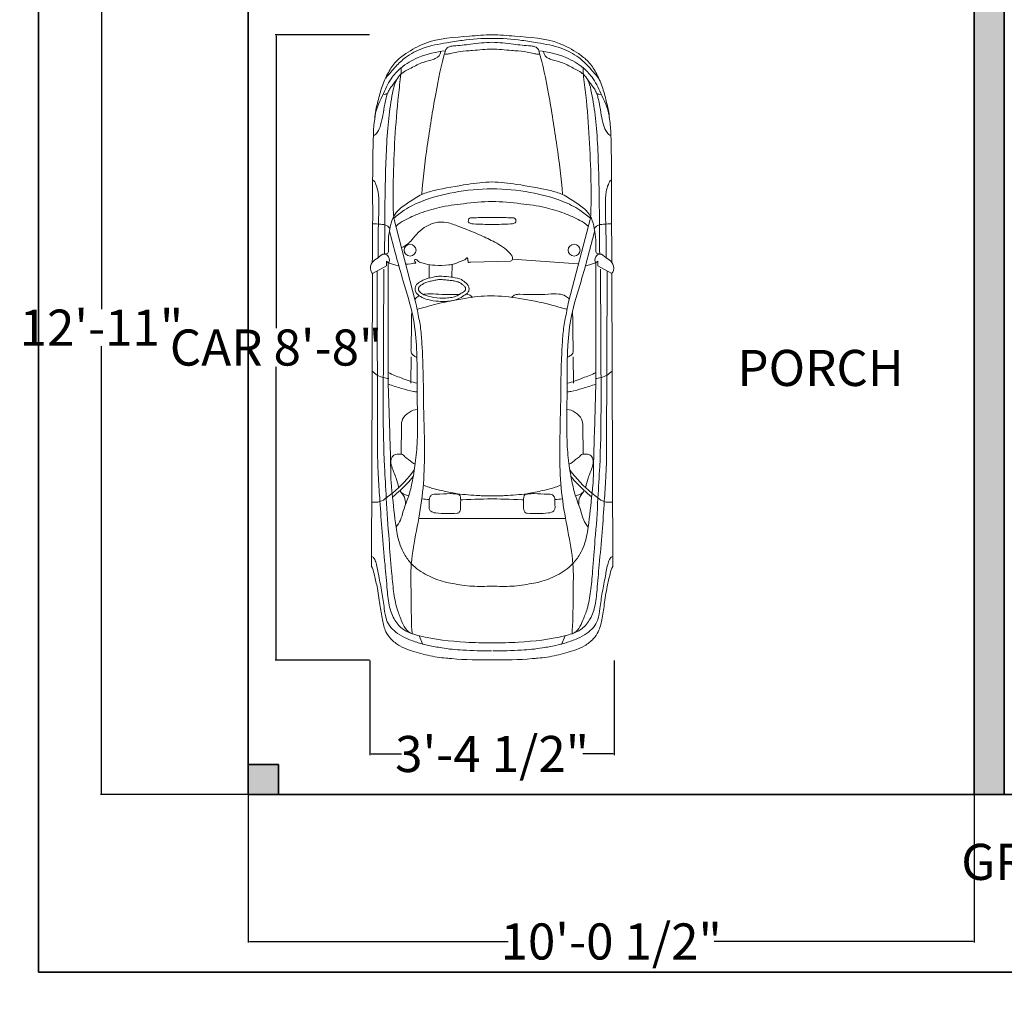
# Model space of a CAD drawing. Units: inches. Extents: x 717 to 1167, y 2046 to 2594.
# Tile 1 of 6: x 717 to 880, y 2046 to 2208. Entities that reach past the tile are written whole.
import ezdxf

# ---------------------------------------------------------------- set-up
doc = ezdxf.new("R2010")
doc.units = ezdxf.units.IN
doc.header["$MEASUREMENT"] = 0
for name, color, linetype, lineweight in [('A-ANNO-DIMS', 2, 'Continuous', 18), ('A-ANNO-TEXT', 7, 'Continuous', 25), ('A-ANNO-TTLB', 7, 'Continuous', 35), ('A-AREA-IDEN', 7, 'Continuous', 18), ('A-COLS', 7, 'Continuous', 35), ('A-COLS-PATT', 140, 'Continuous', 13), ('A-EQPM-VEHI', 8, 'Continuous', 18), ('A-WALL', 7, 'Continuous', 35), ('A-WALL-PATT', 140, 'Continuous', 13)]:
    doc.layers.add(name, color=color, linetype=linetype, lineweight=lineweight)
doc.styles.get("Standard").update_dxf_attribs({"font": 'arial.ttf'})
doc.dimstyles.get("Standard").update_dxf_attribs({"dimtxt": 6, "dimasz": 0.18, "dimexe": 0.18, "dimexo": 0.0625, "dimgap": 0.09, "dimtad": 0, "dimtih": 1, "dimtoh": 1, "dimdec": 1, "dimzin": 0, "dimdsep": 46, "dimlunit": 3, "dimtxsty": 'Standard', "dimcen": 0.09, "dimadec": 0, "dimazin": 0, "dimtfac": 1, "dimtdec": 1, "dimtofl": 0, "dimtmove": 0, "dimatfit": 3, "dimfxl": 1, "dimtolj": 1, "dimtzin": 0, "dimarcsym": 0})

# ---------------------------------------------------------------- blocks, each defined once
blk = doc.blocks.new('A$C242571DA')
for p, q in [((1659.9, 1632), (1714.3, 1732.5)), ((1699.9, 1699.4), (2984.7, 1695.8)), ((1714.3, 1732.5), (3817.1, 1739.9)), ((1638.3, 1618.5), (1625.1, 1632)), ((1625.1, 1632), (1659.9, 1632)), ((1681.8, 1651.6), (2695.2, 1655.3)), ((1317.4, 1579.7), (1909.8, 1424.9)), ((1638.3, 1618.5), (2503.3, 1618.5)), ((1659.9, 1548.1), (1638.3, 1618.5)), ((2503.3, 1618.5), (2861.6, 1607.5)), ((1644, 1489.1), (1610.4, 1020.2)), ((3007.2, 1526.5), (2808.1, 1525.2)), ((2311.9, 1454.3), (2500.6, 1456.9)), ((3474.6, 1401.1), (3474.6, 843)), ((4315.2, 1398), (4377.3, 1370.5)), ((1626.1, 1006.5), (1632.8, 719.7)), ((3474.6, 345.6), (3474.6, 903.8)), ((1740.2, 584.9), (1649.3, 586.9)), ((1746.1, 420.6), (1649.3, 420.6)), ((4315.2, 348.7), (4377.3, 376.3)), ((1317.4, 167), (1909.8, 321.9)), ((2311.9, 292.5), (2500.6, 289.8)), ((3007.2, 220.3), (2808.1, 221.6)), ((1659.9, 198.7), (1638.3, 128.2)), ((1638.3, 128.2), (1625.1, 114.7)), ((1625.1, 114.7), (1659.9, 114.7)), ((1638.3, 128.2), (2503.3, 128.2)), ((1659.9, 114.7), (1714.3, 14.2)), ((1681.8, 95.1), (2695.2, 91.4)), ((2503.3, 128.2), (2861.6, 139.2)), ((1699.9, 47.3), (2984.7, 51)), ((1714.3, 14.2), (3817.1, 6.9))]:
    blk.add_line(p, q)
for centre in [(1546.4, 1462.5), (1546.4, 284.2)]:
    blk.add_ellipse(centre, major_axis=(0, 42.9), ratio=0.983266, start_param=4.712389, end_param=10.995574)
for points, knots in [([(0, 873.4), (0, 927.8), (15.6, 1088.6), (25.5, 1309.8), (120.7, 1476.4), (189.2, 1569), (273.5, 1623.1), (369.9, 1666.3), (483, 1694.7), (561.3, 1714.9), (604.6, 1715.7)], [0, 0, 0, 0, 0.16039, 0.479033, 0.632967, 0.722015, 0.817474, 0.927562, 1.03733, 1.167094, 1.167094, 1.167094, 1.167094]), ([(604.6, 1715.7), (545.5, 1714.5), (448.5, 1664.6), (320.8, 1610.6), (225.4, 1521.2), (147.3, 1390.5), (121.7, 1275.2), (113.6, 1208.7)], [0, 0, 0, 0, 0.1772572, 0.3124951, 0.4151678, 0.5597243, 0.7575412, 0.7575412, 0.7575412, 0.7575412]), ([(722.7, 1726.6), (720.8, 1714.9), (694.5, 1689.9), (643, 1671.8), (573.6, 1655.4), (508.5, 1647), (455.2, 1634.7), (428.7, 1627.3), (416.9, 1624.1)], [0, 0, 0, 0, 0.034703, 0.0959761, 0.1659336, 0.2471559, 0.2929944, 0.3295918, 0.3295918, 0.3295918, 0.3295918]), ([(604.6, 1715.7), (642.1, 1723.4), (788.5, 1729.2), (1039.3, 1732.2), (1344.5, 1729.9), (1542, 1733.1), (1633.8, 1733.7)], [0, 0, 0, 0, 0.114897, 0.437061, 0.754269, 1.029686, 1.029686, 1.029686, 1.029686]), ([(1043.6, 1729.2), (1048.6, 1717.9), (1080.9, 1704.2), (1138.6, 1687.6), (1237.7, 1685.6), (1394.7, 1691.3), (1521.7, 1692.4), (1601.5, 1692.7)], [0, 0, 0, 0, 0.0364992, 0.0923739, 0.1867837, 0.3273982, 0.5667068, 0.5667068, 0.5667068, 0.5667068]), ([(1356.8, 1732.2), (1357.1, 1712.8), (1360, 1678.8), (1363.9, 1630.5), (1383.3, 1613.5), (1391, 1607.2)], [0, 0, 0, 0, 1.462159, 2.651105, 3.386321, 3.386321, 3.386321, 3.386321]), ([(1714.3, 1732.5), (1707.7, 1737.6), (1683.3, 1753), (1628.7, 1741.2), (1605.6, 1691.5), (1561.7, 1652.4), (1594.1, 1610.3), (1627.9, 1608.3), (1638.3, 1618.5)], [0, 0, 0, 0, 0.024864, 0.0846267, 0.1362471, 0.1900683, 0.2245199, 0.2681841, 0.2681841, 0.2681841, 0.2681841]), ([(2414.7, 1735), (2424.9, 1723.3), (2447.2, 1698.8), (2461.2, 1657.6), (2468.1, 1629), (2468, 1616.1)], [1.808086, 1.808086, 1.808086, 1.808086, 2.918874, 4.131288, 5.10151, 5.10151, 5.10151, 5.10151]), ([(3356.5, 1739.4), (3354.9, 1719.2), (3360.8, 1678.2), (3324, 1631.5), (3255.4, 1544.3), (3187.1, 1476.2), (3125.2, 1432.2)], [0, 0, 0, 0, 0.0597371, 0.1139981, 0.1672498, 0.3938869, 0.3938869, 0.3938869, 0.3938869]), ([(3745.3, 1736.8), (3748.5, 1730.1), (3764.2, 1717.1), (3811.5, 1698.6), (3894.7, 1686.7), (4002.9, 1663.2), (4107.9, 1648.7), (4195.8, 1638.3), (4258.6, 1603.2), (4302.1, 1549.7), (4339.9, 1483.8), (4365.2, 1407.6), (4389.6, 1324.4), (4397.9, 1266.9), (4401.8, 1235.2)], [0, 0, 0, 0, 0.0219205, 0.0572122, 0.1522539, 0.2718866, 0.3894011, 0.4710097, 0.5346344, 0.5986698, 0.6733118, 0.758696, 0.8351341, 0.9293726, 0.9293726, 0.9293726, 0.9293726]), ([(3817.1, 1739.9), (3833.2, 1729.7), (3882.9, 1718.2), (3973.3, 1695.2), (4085.1, 1680.5), (4193.8, 1662.8), (4280.6, 1644.3), (4343.9, 1598.1), (4390, 1540.3), (4427.4, 1448.7), (4457.8, 1336.6), (4475.7, 1233.4), (4478.4, 1175.1), (4479.3, 1161.6)], [0, 0, 0, 0, 0.056668, 0.14946, 0.28161, 0.392935, 0.481686, 0.542967, 0.622845, 0.69797, 0.833643, 0.965665, 1.00577, 1.00577, 1.00577, 1.00577]), ([(310.7, 1637.3), (282.5, 1613.7), (230.1, 1569.9), (148.7, 1486.2), (84.8, 1361.3), (60, 1219), (32.6, 1054.3), (25.1, 944.9), (25.1, 873.4)], [0, 0, 0, 0, 0.1095129, 0.2035347, 0.3452507, 0.5161382, 0.6275464, 0.8383798, 0.8383798, 0.8383798, 0.8383798]), ([(426.8, 1656.7), (428.5, 1646.6), (426.9, 1625), (399.8, 1616.6), (368.1, 1593.9), (328, 1564.6), (271.6, 1523.9), (237, 1451.9), (196.2, 1376.7), (183.8, 1314.9), (170, 1279.6), (157.2, 1254.2), (133.3, 1244.4), (118.6, 1242.9)], [0, 0, 0, 0, 0.0304541, 0.0502818, 0.0786089, 0.1479133, 0.1986294, 0.2831705, 0.3780326, 0.4523267, 0.4667809, 0.4902599, 0.5347198, 0.5347198, 0.5347198, 0.5347198]), ([(323.7, 1557.5), (344.8, 1571.9), (400.4, 1585.1), (516, 1606.8), (680.3, 1625.8), (885.4, 1635.7), (1116.8, 1642.2), (1346.1, 1644.2), (1504.7, 1644.7), (1574, 1645.7)], [0, 0, 0, 0, 0.076148, 0.165903, 0.355672, 0.569871, 0.782325, 1.050047, 1.257936, 1.257936, 1.257936, 1.257936]), ([(1574, 1645.7), (1572.9, 1638), (1574.1, 1622), (1559.9, 1618.7), (1555.2, 1617.8)], [0, 0, 0, 0, 0.02274132, 0.03717479, 0.03717479, 0.03717479, 0.03717479]), ([(2695.2, 1655.3), (2829.9, 1655.3), (3041.2, 1651.4), (3351.3, 1630.7), (3527.5, 1623.2), (3626.6, 1612)], [0, 0, 0, 0, 0.4042759, 0.6333827, 0.9326252, 0.9326252, 0.9326252, 0.9326252]), ([(2984.7, 1695.8), (3051, 1695.6), (3172.1, 1691.3), (3367.4, 1677.6), (3575.2, 1664.3), (3788.2, 1643.6), (3968, 1628.1), (4103.8, 1616.8), (4203.6, 1578.1), (4271.8, 1519.5), (4300.6, 1452.1), (4341.7, 1305.3), (4361.8, 1111.2), (4367.5, 936.8), (4367.5, 873.4)], [0, 0, 0, 0, 0.198873, 0.363323, 0.587433, 0.823543, 1.004622, 1.129816, 1.230113, 1.320655, 1.388577, 1.443334, 1.771447, 1.958652, 1.958652, 1.958652, 1.958652]), ([(1317.4, 1579.7), (1227.8, 1586.1), (1036, 1584.8), (741.2, 1572.5), (486.1, 1553.3), (333.3, 1534.3), (283.3, 1528.5)], [0, 0, 0, 0, 0.269375, 0.574535, 0.885339, 1.036319, 1.036319, 1.036319, 1.036319]), ([(1555.2, 1617.8), (1527.7, 1617.8), (1472.5, 1620.4), (1392.7, 1608.8), (1318.5, 1591), (1249.4, 1545.5), (1201.4, 1466.7), (1142.8, 1385.7), (1104.8, 1240.4), (1076, 1072.3), (1056.4, 932.4), (1056.4, 873.4)], [0, 0, 0, 0, 0.082256, 0.165174, 0.241383, 0.30939, 0.405348, 0.511507, 0.603349, 0.843635, 1.017671, 1.017671, 1.017671, 1.017671]), ([(1317.4, 1579.7), (1296.6, 1555.5), (1247.9, 1494.4), (1177.6, 1350.5), (1124.2, 1137.4), (1105.5, 964.9), (1105.5, 873.4)], [0, 0, 0, 0, 0.0947759, 0.2311242, 0.4700259, 0.7400315, 0.7400315, 0.7400315, 0.7400315]), ([(1372.8, 1563.1), (1357.2, 1545), (1321.6, 1490.1), (1277, 1385.7), (1232.8, 1244.2), (1211.1, 1069.4), (1196.8, 942.4), (1196.8, 873.4)], [0, 0, 0, 0, 0.0708922, 0.1925846, 0.3348457, 0.5072814, 0.7109928, 0.7109928, 0.7109928, 0.7109928]), ([(3535.9, 1563.1), (3520.1, 1550.9), (3484.4, 1526.1), (3408.2, 1510.9), (3323.4, 1473.1), (3207.9, 1445), (3072.6, 1422.2), (2866.9, 1404.6), (2626.4, 1412.9), (2396.7, 1410.8), (2200.9, 1416.9), (2001.3, 1438.2), (1732.1, 1525.9), (1527.9, 1578.9), (1407.5, 1610.7)], [0, 0, 0, 0, 0.05975, 0.126928, 0.230034, 0.336675, 0.482225, 0.641324, 0.954906, 1.203173, 1.330375, 1.542773, 1.802261, 2.175545, 2.175545, 2.175545, 2.175545]), ([(2424, 1618.7), (2441.5, 1589.9), (2464.2, 1518.9), (2495.4, 1450.9), (2501.6, 1411.3)], [0, 0, 0, 0, 0.1000351, 0.2184418, 0.2184418, 0.2184418, 0.2184418]), ([(2507.7, 1618.4), (2521, 1587.7), (2536.6, 1527.1), (2559.6, 1458.5), (2563.3, 1420.6), (2563.8, 1411.4)], [0, 0, 0, 0, 2.528586, 4.711885, 5.408215, 5.408215, 5.408215, 5.408215]), ([(2861.6, 1607.5), (2921.1, 1607.3), (3047.2, 1600.8), (3191.4, 1602), (3356.6, 1584.1), (3498.3, 1570.6), (3623.2, 1549.4), (3664.1, 1533.3)], [0, 0, 0, 0, 0.1783018, 0.3787173, 0.431954, 0.6762374, 0.8077184, 0.8077184, 0.8077184, 0.8077184]), ([(3248.1, 1545.2), (3226.9, 1550.4), (3176.1, 1562.1), (3113.7, 1592.9), (3052.6, 1605.3), (3010.4, 1578.8), (3010.3, 1545.3), (3010.3, 1515.9), (3033.7, 1500.1), (3052.6, 1465.2), (3078.9, 1443.5), (3084, 1424.4)], [0, 0, 0, 0, 0.0655106, 0.1550445, 0.2094604, 0.2438604, 0.287164, 0.3001388, 0.3275984, 0.3616951, 0.4200969, 0.4200969, 0.4200969, 0.4200969]), ([(3319, 1587.1), (3303.3, 1568.1), (3256.9, 1516.7), (3206.7, 1467.3), (3171.4, 1439.5)], [0, 0, 0, 0, 1.868162, 5.271297, 5.271297, 5.271297, 5.271297]), ([(3626.6, 1612), (3702.5, 1609.1), (3826.2, 1596.8), (3991.4, 1583.2), (4111.7, 1562.4), (4212.2, 1522.7), (4290.4, 1488), (4300.7, 1447.5)], [0, 0, 0, 0, 0.2277977, 0.3719478, 0.4996814, 0.5863441, 0.709615, 0.709615, 0.709615, 0.709615]), ([(2808.1, 1525.2), (2791.9, 1525.1), (2751.9, 1519.7), (2710.6, 1472.6), (2690, 1431.1), (2690.5, 1409.6)], [0, 0, 0, 0, 0.0486628, 0.1144515, 0.1777721, 0.1777721, 0.1777721, 0.1777721]), ([(3275.5, 1532.8), (3287.5, 1528.3), (3299.8, 1504.9), (3308.4, 1482.5), (3311.7, 1472.6)], [0, 0, 0, 0, 0.983949, 1.771691, 1.771691, 1.771691, 1.771691]), ([(3372.2, 1495.3), (3354.4, 1496.8), (3316, 1494.7), (3291.6, 1525.8), (3275.5, 1532.8)], [0, 0, 0, 0, 0.0535488, 0.1060573, 0.1060573, 0.1060573, 0.1060573]), ([(3664.1, 1533.3), (3687, 1526), (3734.8, 1502.3), (3816.7, 1444.8), (3884.1, 1342.9), (3925.1, 1239.9), (3937.3, 1177), (3940.4, 1157.6)], [0, 0, 0, 0, 0.0720749, 0.1581284, 0.2958089, 0.4262456, 0.4842292, 0.4842292, 0.4842292, 0.4842292]), ([(1898.5, 1426.2), (1889, 1420.6), (1871, 1397.2), (1856.4, 1345.2), (1867.7, 1233.5), (1864.3, 1132.3), (1863, 1038.5), (1876.9, 1022.3), (1884.5, 1015.7)], [0, 0, 0, 0, 0.842998, 2.122875, 3.997599, 9.174838, 10.012722, 10.751336, 10.751336, 10.751336, 10.751336]), ([(1909.8, 1424.9), (1933.5, 1418.7), (1995.6, 1407.6), (2094.4, 1385.8), (2211.8, 1377.1), (2419, 1366.9), (2704.7, 1366.5), (3032.7, 1354.2), (3316.2, 1371), (3558.7, 1415.9), (3789.1, 1461.7), (4028.9, 1452.9), (4196.2, 1455.2), (4292.7, 1447.9), (4300.7, 1447.5)], [0, 0, 0, 0, 0.073325, 0.188896, 0.303039, 0.425821, 0.811242, 1.159737, 1.41058, 1.660623, 1.899627, 2.11145, 2.377727, 2.401703, 2.401703, 2.401703, 2.401703]), ([(1997.2, 1450.5), (2039.7, 1454.5), (2126.7, 1451.9), (2219.8, 1454.5), (2287.1, 1456.9), (2305.7, 1434.4), (2313.2, 1419.9), (2315.8, 1413.5)], [0, 0, 0, 0, 3.267856, 6.568708, 7.399663, 8.099385, 8.621705, 8.621705, 8.621705, 8.621705]), ([(113.6, 1208.7), (215.2, 1238.6), (443.2, 1284.9), (788, 1338.7), (1029.5, 1370.7), (1146.4, 1378.6)], [0, 0, 0, 0, 0.317374, 0.69576, 1.04714, 1.04714, 1.04714, 1.04714]), ([(1969.6, 1407.3), (1960.5, 1369.8), (1927, 1259.1), (1890.9, 1078.4), (1874.3, 933), (1874.3, 864.4)], [0, 0, 0, 0, 0.1139079, 0.3411539, 0.543502, 0.543502, 0.543502, 0.543502]), ([(3231.5, 1368.3), (3240.8, 1356.2), (3253.1, 1315.7), (3271.9, 1240.7), (3297.9, 1127.9), (3310.5, 974.6), (3311.2, 858.3), (3311.6, 794.4)], [0, 0, 0, 0, 0.0451009, 0.1211996, 0.2308505, 0.385263, 0.5739042, 0.5739042, 0.5739042, 0.5739042]), ([(3294.8, 1174.5), (3294.8, 1207.4), (3299.6, 1249.5), (3298.3, 1303.9), (3326.3, 1329), (3363.9, 1320.7), (3399.3, 1329.3), (3422.1, 1315.7), (3430.7, 1297.9), (3438.7, 1234.2), (3439.6, 1174.4), (3434.7, 1112.2), (3418.9, 1102), (3395.9, 1098.6), (3362.6, 1100.9), (3331.1, 1096.6), (3298.8, 1107.6), (3297.3, 1140.3), (3294.8, 1160.9), (3294.8, 1174.5)], [0, 0, 0, 0, 0.0969044, 0.1295913, 0.1506192, 0.1985921, 0.2360698, 0.2557908, 0.2719711, 0.2929882, 0.44406, 0.4519132, 0.4720918, 0.4918599, 0.5228758, 0.5707096, 0.5892096, 0.6145759, 0.654681, 0.654681, 0.654681, 0.654681]), ([(113.6, 1208.7), (103.3, 1207), (83.6, 1187.6), (76.5, 1122.2), (68.2, 1017.3), (53.4, 925), (53.4, 873.4)], [0, 0, 0, 0, 0.0314754, 0.0702057, 0.1915753, 0.3439346, 0.3439346, 0.3439346, 0.3439346]), ([(135.5, 1213.1), (139.1, 1211.8), (138.4, 1193.3), (132.6, 1168.3), (118.8, 1111.9), (115.6, 1058.9), (109, 974.6), (102.4, 920.1), (102.4, 873.4)], [0, 0, 0, 0, 0.0114788, 0.0403472, 0.0875838, 0.1755608, 0.1991501, 0.3369659, 0.3369659, 0.3369659, 0.3369659]), ([(4401.8, 1235.2), (4411.9, 1185.3), (4421.6, 1065.8), (4424.1, 946.5), (4424.1, 878)], [0, 0, 0, 0, 0.1502861, 0.3522699, 0.3522699, 0.3522699, 0.3522699]), ([(3940.4, 1157.6), (3949.9, 1111), (3964.3, 1016.4), (3960.5, 921), (3959.8, 873.4)], [0, 0, 0, 0, 0.140379, 0.2808468, 0.2808468, 0.2808468, 0.2808468]), ([(3339.2, 1099), (3339.1, 1094.8), (3336.4, 1010.6), (3333.2, 926.3), (3330, 846.2)], [11.235438, 11.235438, 11.235438, 11.235438, 11.552536, 17.586883, 17.586883, 17.586883, 17.586883]), ([(1311.3, 873.4), (1311.2, 902.4), (1309.2, 950.9), (1315, 1002.2), (1314.2, 1039.4), (1332.1, 1044.9), (1345.7, 1044.2), (1356.8, 1028.5), (1359.2, 970.2), (1361.5, 917.6), (1362.9, 873.4)], [0, 0, 0, 0, 0.0857277, 0.1381048, 0.1641986, 0.1769751, 0.1890325, 0.2028129, 0.2286049, 0.3592554, 0.3592554, 0.3592554, 0.3592554]), ([(1626.1, 1006.5), (1623.5, 1013), (1603.1, 1029.4), (1559.1, 995), (1523, 951.9), (1480.3, 878.3), (1430.5, 774.3), (1385.5, 658.5), (1343.7, 551.3), (1343, 461.7), (1380.3, 386.9), (1428.2, 329.9), (1480.1, 294.6), (1509.8, 257.4), (1524.8, 232.6), (1528, 222.1)], [0, 0, 0, 0, 0.527288, 1.647451, 3.487558, 5.099073, 7.968657, 12.238313, 14.475187, 16.613757, 18.744202, 20.639343, 22.223389, 23.452731, 24.286529, 24.286529, 24.286529, 24.286529]), ([(3231.5, 378.5), (3240.8, 390.5), (3253.1, 431), (3271.9, 506.1), (3297.9, 618.9), (3310.5, 772.1), (3311.2, 888.4), (3311.6, 952.4)], [0, 0, 0, 0, 0.0451009, 0.1211996, 0.2308505, 0.385263, 0.5739042, 0.5739042, 0.5739042, 0.5739042]), ([(0, 873.4), (0, 819), (15.6, 658.1), (25.5, 437), (120.7, 270.3), (189.2, 177.8), (273.5, 123.7), (369.9, 80.4), (483, 52), (561.3, 31.9), (604.6, 31)], [0, 0, 0, 0, 0.16039, 0.479033, 0.632967, 0.722015, 0.817474, 0.927562, 1.03733, 1.167094, 1.167094, 1.167094, 1.167094]), ([(310.7, 109.5), (282.5, 133.1), (230.1, 176.9), (148.7, 260.5), (84.8, 385.5), (60, 527.8), (32.6, 692.4), (25.1, 801.9), (25.1, 873.4)], [0, 0, 0, 0, 0.1095129, 0.2035347, 0.3452507, 0.5161382, 0.6275464, 0.8383798, 0.8383798, 0.8383798, 0.8383798]), ([(113.6, 538.1), (103.3, 539.8), (83.6, 559.2), (76.5, 624.5), (68.2, 729.4), (53.4, 821.7), (53.4, 873.4)], [0, 0, 0, 0, 0.0314754, 0.0702057, 0.1915753, 0.3439346, 0.3439346, 0.3439346, 0.3439346]), ([(135.5, 533.6), (139.1, 534.9), (138.4, 553.4), (132.6, 578.4), (118.8, 634.9), (115.6, 687.8), (109, 772.2), (102.4, 826.7), (102.4, 873.4)], [0, 0, 0, 0, 0.0114788, 0.0403472, 0.0875838, 0.1755608, 0.1991501, 0.3369659, 0.3369659, 0.3369659, 0.3369659]), ([(1555.2, 129), (1527.7, 129), (1472.5, 126.3), (1392.7, 138), (1318.5, 155.7), (1249.4, 201.3), (1201.4, 280.1), (1142.8, 361.1), (1104.8, 506.4), (1076, 674.5), (1056.4, 814.4), (1056.4, 873.4)], [0, 0, 0, 0, 0.082256, 0.165174, 0.241383, 0.30939, 0.405348, 0.511507, 0.603349, 0.843635, 1.017671, 1.017671, 1.017671, 1.017671]), ([(1317.4, 167), (1296.6, 191.2), (1247.9, 252.4), (1177.6, 396.3), (1124.2, 609.4), (1105.5, 781.8), (1105.5, 873.4)], [0, 0, 0, 0, 0.0947759, 0.2311242, 0.4700259, 0.7400315, 0.7400315, 0.7400315, 0.7400315]), ([(1372.8, 183.6), (1357.2, 201.8), (1321.6, 256.7), (1277, 361), (1232.8, 502.6), (1211.1, 677.3), (1196.8, 804.3), (1196.8, 873.4)], [0, 0, 0, 0, 0.0708922, 0.1925846, 0.3348457, 0.5072814, 0.7109928, 0.7109928, 0.7109928, 0.7109928]), ([(1311.3, 873.4), (1311.2, 844.3), (1309.2, 795.8), (1315, 744.6), (1314.2, 707.4), (1332.1, 701.9), (1345.7, 702.6), (1356.8, 718.2), (1359.2, 776.6), (1361.5, 829.1), (1362.9, 873.4)], [0, 0, 0, 0, 0.0857277, 0.1381048, 0.1641986, 0.1769751, 0.1890325, 0.2028129, 0.2286049, 0.3592554, 0.3592554, 0.3592554, 0.3592554]), ([(1969.6, 339.5), (1960.5, 377), (1926.9, 487.6), (1892.9, 662.7), (1874.3, 801.8), (1874.3, 864.4)], [0, 0, 0, 0, 0.1139079, 0.3411539, 0.5260188, 0.5260188, 0.5260188, 0.5260188]), ([(2984.7, 51), (3051, 51.1), (3172.1, 55.5), (3367.4, 69.2), (3575.2, 82.5), (3788.2, 103.1), (3968, 118.7), (4103.8, 130), (4203.6, 168.6), (4271.8, 227.3), (4300.6, 294.7), (4341.7, 441.5), (4361.8, 635.5), (4367.5, 809.9), (4367.5, 873.4)], [0, 0, 0, 0, 0.198873, 0.363323, 0.587433, 0.823543, 1.004622, 1.129816, 1.230113, 1.320655, 1.388577, 1.443334, 1.771447, 1.958652, 1.958652, 1.958652, 1.958652]), ([(3339.2, 647.8), (3339.1, 652), (3336.4, 736.2), (3333.2, 820.5), (3330, 900.6)], [11.235438, 11.235438, 11.235438, 11.235438, 11.552536, 17.586883, 17.586883, 17.586883, 17.586883]), ([(3940.4, 589.1), (3949.9, 635.7), (3964.3, 730.4), (3960.5, 825.8), (3959.8, 873.4)], [0, 0, 0, 0, 0.140379, 0.2808468, 0.2808468, 0.2808468, 0.2808468]), ([(4401.8, 511.5), (4411.9, 561.5), (4421.6, 681), (4424.1, 800.3), (4424.1, 868.8)], [0, 0, 0, 0, 0.1502861, 0.3522699, 0.3522699, 0.3522699, 0.3522699]), ([(1639.2, 326.1), (1635.3, 323.6), (1629, 318.4), (1613.1, 314.9), (1612, 324.2), (1613.2, 330.4), (1619, 337.5), (1629, 345.7), (1637.9, 366.1), (1649, 404.8), (1656.3, 472.9), (1656.2, 543.1), (1644.6, 610.9), (1623, 651.2), (1615, 684.3), (1598.5, 691.2), (1604, 696.6), (1610.3, 699.7), (1618.8, 698.9), (1625.9, 701.3), (1638.1, 698.6), (1633, 713.4), (1632.8, 719.7)], [0, 0, 0, 0, 0.0138597, 0.0278304, 0.0329137, 0.0379971, 0.0465756, 0.0592704, 0.0762214, 0.1105991, 0.1789801, 0.2766959, 0.3173629, 0.3800771, 0.4110544, 0.4160421, 0.4210284, 0.4277212, 0.4387433, 0.4448131, 0.4508005, 0.4694463, 0.4694463, 0.4694463, 0.4694463]), ([(1740.2, 584.9), (1737.8, 571.7), (1749.5, 644.3), (1766.4, 664.5), (1792.2, 700.2), (1821.5, 709.7), (1853.1, 703.9), (1874, 668.4), (1904.5, 622.6), (1915.6, 557.2), (1915.1, 484.2), (1905.7, 417.6), (1884.9, 362.8), (1859.3, 329.1), (1831.3, 318.1), (1810.8, 322.7), (1792.2, 329.3), (1777.9, 350.3), (1753, 385.9), (1737.9, 465.8), (1728.8, 497.3), (1742.4, 597.6), (1740.2, 584.9)], [0, 0, 0, 0, 0.03969, 0.089634, 0.13125, 0.1542862, 0.1797268, 0.2207266, 0.2680991, 0.3447665, 0.4095645, 0.4843001, 0.541515, 0.5817687, 0.6060665, 0.6262474, 0.6436722, 0.6634686, 0.6988791, 0.7758465, 0.8696394, 0.907731, 0.907731, 0.907731, 0.907731]), ([(1863.4, 685.6), (1863.6, 693.5), (1865.3, 711), (1876.9, 724.5), (1884.5, 731)], [9.436432, 9.436432, 9.436432, 9.436432, 10.012722, 10.751336, 10.751336, 10.751336, 10.751336]), ([(1764.9, 587), (1765.6, 590.8), (1766.4, 595.5), (1768.5, 605.7), (1769.7, 611.3), (1773.4, 626.6), (1775.6, 633), (1779.7, 642.1), (1781.6, 644.9), (1785.7, 650.6), (1787.1, 652.5), (1793, 660.3), (1797.4, 666.2), (1804.2, 673.7), (1806.8, 676.1), (1811.1, 679.4), (1812.9, 680.5), (1816.8, 682.1), (1818.8, 682.7), (1824.4, 683.5), (1828.3, 683.2), (1832.5, 682), (1833.6, 681.5), (1836, 680.2), (1837.9, 678.7), (1842.4, 673.7), (1844.9, 670.1), (1850.3, 661.7), (1853.4, 656.6), (1859.3, 647.3), (1862.1, 642.8), (1868.3, 632.6), (1871.4, 626.9), (1876.7, 615.7), (1878.9, 609.8), (1882.8, 597.4), (1884.4, 590.8), (1888.3, 570.5), (1889.7, 556.1), (1891.2, 527.4), (1891.1, 513.1), (1888.9, 470), (1885.1, 441.2), (1874.3, 404), (1870.6, 393.8), (1863.5, 378.7), (1860.6, 373.4), (1854.4, 363.6), (1851.2, 359.2), (1845, 352.6), (1842, 350.2), (1835.8, 346.4), (1832.6, 345.3), (1828.8, 344.6), (1827.9, 344.6), (1824.6, 344.9), (1822.6, 345.2), (1817.8, 346.4), (1814.9, 347.3), (1810.9, 348.7), (1809.4, 349.4), (1808.3, 350.1), (1808.1, 350.2), (1807.3, 351), (1806.7, 351.6), (1804.7, 354), (1803.1, 356.2), (1799.6, 361.3), (1798, 363.7), (1794.9, 368.2), (1793.4, 370.4), (1789.2, 376.9), (1786.7, 381), (1782.4, 389.3), (1780.5, 393.6), (1776.9, 403), (1775.2, 408), (1770.7, 423.5), (1768.3, 434.2), (1764.9, 450.5), (1763.6, 456.4), (1761.4, 466.8), (1760.4, 471.4), (1758.1, 484.4), (1757.3, 492.6), (1757.5, 510.7), (1757.8, 516.5), (1758.6, 528.4), (1759.1, 534.3), (1761.1, 553.9), (1763.1, 570.6), (1764.4, 581.5), (1764.6, 583), (1764.7, 585), (1764.8, 585.5), (1764.8, 586.5), (1764.8, 586.7), (1764.9, 587)], [0.497033, 0.497033, 0.497033, 0.497033, 0.723444, 0.723444, 0.974636, 0.974636, 1.50964, 1.50964, 2.044645, 2.044645, 2.271061, 2.271061, 2.862376, 2.862376, 3.217654, 3.217654, 3.537253, 3.537253, 3.856852, 3.856852, 4.368613, 4.368613, 4.584627, 4.584627, 4.99269, 4.99269, 5.400753, 5.400753, 5.808816, 5.808816, 6.216879, 6.216879, 6.778716, 6.778716, 7.350371, 7.350371, 7.922025, 7.922025, 9.065335, 9.065335, 10.208644, 10.208644, 12.495263, 12.495263, 13.409896, 13.409896, 13.929088, 13.929088, 14.44828, 14.44828, 14.909885, 14.909885, 15.371489, 15.371489, 15.62524, 15.62524, 15.87899, 15.87899, 16.120875, 16.120875, 16.36276, 16.36276, 16.51635, 16.51635, 16.669941, 16.669941, 16.921521, 16.921521, 17.136676, 17.136676, 17.351831, 17.351831, 17.782142, 17.782142, 18.204974, 18.204974, 18.627807, 18.627807, 19.473473, 19.473473, 19.978923, 19.978923, 20.484372, 20.484372, 21.475119, 21.475119, 21.859144, 21.859144, 22.162884, 22.162884, 22.770362, 22.770362, 22.900493, 22.900493, 22.951221, 22.951221, 22.964298, 22.964298, 22.964298, 22.964298]), ([(1863.7, 379.4), (1862.6, 384.2), (1857.6, 413.7), (1866.5, 501.6), (1865.2, 581.4), (1864.1, 639.5)], [1.749253, 1.749253, 1.749253, 1.749253, 2.122875, 3.997599, 8.307432, 8.307432, 8.307432, 8.307432]), ([(3294.8, 572.3), (3294.8, 539.4), (3299.6, 497.2), (3298.3, 442.9), (3326.3, 417.8), (3363.9, 426), (3399.3, 417.5), (3422.1, 431), (3430.7, 448.9), (3438.7, 512.5), (3439.6, 572.4), (3434.7, 634.6), (3418.9, 644.7), (3395.9, 648.2), (3362.6, 645.9), (3331.1, 650.1), (3298.8, 639.2), (3297.3, 606.5), (3294.8, 585.9), (3294.8, 572.3)], [0, 0, 0, 0, 0.0969044, 0.1295913, 0.1506192, 0.1985921, 0.2360698, 0.2557908, 0.2719711, 0.2929882, 0.44406, 0.4519132, 0.4720918, 0.4918599, 0.5228758, 0.5707096, 0.5892096, 0.6145759, 0.654681, 0.654681, 0.654681, 0.654681]), ([(3664.1, 213.5), (3687, 220.8), (3734.8, 244.4), (3816.7, 302), (3884.1, 403.8), (3925.1, 506.9), (3937.3, 569.7), (3940.4, 589.1)], [0, 0, 0, 0, 0.0720749, 0.1581284, 0.2958089, 0.4262456, 0.4842292, 0.4842292, 0.4842292, 0.4842292]), ([(3817.1, 6.9), (3833.2, 17), (3882.9, 28.6), (3973.3, 51.5), (4085.1, 66.3), (4193.8, 84), (4280.6, 102.4), (4343.9, 148.6), (4390, 206.4), (4427.4, 298), (4457.8, 410.1), (4475.7, 513.3), (4478.4, 571.6), (4479.3, 585.2)], [0, 0, 0, 0, 0.056668, 0.14946, 0.28161, 0.392935, 0.481686, 0.542967, 0.622845, 0.69797, 0.833643, 0.965665, 1.00577, 1.00577, 1.00577, 1.00577]), ([(604.6, 31), (545.5, 32.3), (448.5, 82.2), (320.8, 136.1), (225.4, 225.5), (147.3, 356.2), (121.7, 471.5), (113.6, 538.1)], [0, 0, 0, 0, 0.1772572, 0.3124951, 0.4151678, 0.5597243, 0.7575412, 0.7575412, 0.7575412, 0.7575412]), ([(113.6, 538.1), (215.2, 508.2), (443.2, 461.9), (788, 408.1), (1029.5, 376), (1146.4, 368.2)], [0, 0, 0, 0, 0.317374, 0.69576, 1.04714, 1.04714, 1.04714, 1.04714]), ([(426.8, 90), (428.5, 100.2), (426.9, 121.8), (399.8, 130.1), (368.1, 152.8), (328, 182.2), (271.6, 222.8), (237, 294.9), (196.2, 370.1), (183.8, 431.9), (170, 467.2), (157.2, 492.6), (133.3, 502.4), (118.6, 503.9)], [0, 0, 0, 0, 0.0304541, 0.0502818, 0.0786089, 0.1479133, 0.1986294, 0.2831705, 0.3780326, 0.4523267, 0.4667809, 0.4902599, 0.5347198, 0.5347198, 0.5347198, 0.5347198]), ([(3745.3, 10), (3748.5, 16.7), (3764.2, 29.7), (3811.5, 48.1), (3894.7, 60.1), (4002.9, 83.6), (4107.9, 98), (4195.8, 108.4), (4258.6, 143.5), (4302.1, 197), (4339.9, 262.9), (4365.2, 339.2), (4389.6, 422.4), (4397.9, 479.8), (4401.8, 511.5)], [0, 0, 0, 0, 0.0219205, 0.0572122, 0.1522539, 0.2718866, 0.3894011, 0.4710097, 0.5346344, 0.5986698, 0.6733118, 0.758696, 0.8351341, 0.9293726, 0.9293726, 0.9293726, 0.9293726]), ([(1909.8, 321.9), (1933.5, 328.1), (1995.6, 339.2), (2094.4, 361), (2211.8, 369.6), (2419, 379.8), (2704.7, 380.3), (3032.7, 392.6), (3316.2, 375.8), (3558.7, 330.9), (3789.1, 285.1), (4028.9, 293.9), (4196.2, 291.5), (4292.7, 298.8), (4300.7, 299.2)], [0, 0, 0, 0, 0.073325, 0.188896, 0.303039, 0.425821, 0.811242, 1.159737, 1.41058, 1.660623, 1.899627, 2.11145, 2.377727, 2.401703, 2.401703, 2.401703, 2.401703]), ([(3535.9, 183.7), (3520.1, 195.9), (3484.4, 220.6), (3408.2, 235.8), (3323.4, 273.7), (3207.9, 301.8), (3072.6, 324.6), (2866.9, 342.1), (2626.4, 333.8), (2396.7, 335.9), (2200.9, 329.9), (2001.3, 308.6), (1732.1, 220.8), (1527.9, 167.8), (1407.5, 136)], [0, 0, 0, 0, 0.05975, 0.126928, 0.230034, 0.336675, 0.482225, 0.641324, 0.954906, 1.203173, 1.330375, 1.542773, 1.802261, 2.175545, 2.175545, 2.175545, 2.175545]), ([(1898.5, 320.6), (1889, 326.2), (1880.8, 336.8), (1874.8, 348.3), (1874, 349.7)], [0, 0, 0, 0, 0.8429982, 0.9626806, 0.9626806, 0.9626806, 0.9626806]), ([(1997.2, 296.3), (2039.7, 292.2), (2126.7, 294.9), (2219.8, 292.3), (2287.1, 289.9), (2305.7, 312.3), (2313.2, 326.9), (2315.8, 333.2)], [0, 0, 0, 0, 3.267856, 6.568708, 7.399663, 8.099385, 8.621705, 8.621705, 8.621705, 8.621705]), ([(2424, 128), (2441.5, 156.9), (2464.2, 227.8), (2495.4, 295.8), (2501.6, 335.5)], [0, 0, 0, 0, 0.1000351, 0.2184418, 0.2184418, 0.2184418, 0.2184418]), ([(2507.7, 128.3), (2521, 159.1), (2536.6, 219.7), (2559.6, 288.3), (2563.3, 326.1), (2563.8, 335.3)], [0, 0, 0, 0, 2.528586, 4.711885, 5.408215, 5.408215, 5.408215, 5.408215]), ([(2808.1, 221.6), (2791.9, 221.6), (2751.9, 227.1), (2710.6, 274.2), (2690, 315.7), (2690.5, 337.1)], [0, 0, 0, 0, 0.0486628, 0.1144515, 0.1777721, 0.1777721, 0.1777721, 0.1777721]), ([(3248.1, 201.6), (3226.9, 196.3), (3176.1, 184.7), (3113.7, 153.8), (3052.6, 141.4), (3010.4, 168), (3010.3, 201.5), (3010.3, 230.9), (3033.7, 246.6), (3052.6, 281.6), (3078.9, 303.2), (3084, 322.4)], [0, 0, 0, 0, 0.0655106, 0.1550445, 0.2094604, 0.2438604, 0.287164, 0.3001388, 0.3275984, 0.3616951, 0.4200969, 0.4200969, 0.4200969, 0.4200969]), ([(3356.5, 7.4), (3354.9, 27.5), (3360.8, 68.5), (3324, 115.2), (3255.4, 202.5), (3187.1, 270.5), (3125.2, 314.6)], [0, 0, 0, 0, 0.0597371, 0.1139981, 0.1672498, 0.3938869, 0.3938869, 0.3938869, 0.3938869]), ([(3319, 159.7), (3303.3, 178.6), (3256.9, 230), (3206.7, 279.5), (3171.4, 307.2)], [0, 0, 0, 0, 1.868162, 5.271297, 5.271297, 5.271297, 5.271297]), ([(3626.6, 134.7), (3702.5, 137.7), (3826.2, 149.9), (3991.4, 163.5), (4111.7, 184.4), (4212.2, 224.1), (4290.4, 258.8), (4300.7, 299.2)], [0, 0, 0, 0, 0.2277977, 0.3719478, 0.4996814, 0.5863441, 0.709615, 0.709615, 0.709615, 0.709615]), ([(1317.4, 167), (1227.8, 160.7), (1036, 161.9), (741.2, 174.2), (486.1, 193.4), (333.3, 212.5), (283.3, 218.3)], [0, 0, 0, 0, 0.269375, 0.574535, 0.885339, 1.036319, 1.036319, 1.036319, 1.036319]), ([(2861.6, 139.2), (2921.1, 139.4), (3047.2, 146), (3191.4, 144.8), (3356.6, 162.6), (3498.3, 176.1), (3623.2, 197.4), (3664.1, 213.5)], [0, 0, 0, 0, 0.1783018, 0.3787173, 0.431954, 0.6762374, 0.8077184, 0.8077184, 0.8077184, 0.8077184]), ([(3275.5, 214), (3287.5, 218.5), (3299.8, 241.9), (3308.4, 264.3), (3311.7, 274.2)], [0, 0, 0, 0, 0.983949, 1.771691, 1.771691, 1.771691, 1.771691]), ([(3372.2, 251.5), (3354.4, 249.9), (3316, 252), (3291.6, 220.9), (3275.5, 214)], [0, 0, 0, 0, 0.0535488, 0.1060573, 0.1060573, 0.1060573, 0.1060573]), ([(323.7, 189.2), (344.8, 174.9), (400.4, 161.7), (516, 139.9), (680.3, 121), (885.4, 111), (1116.8, 104.5), (1346.1, 102.5), (1504.7, 102), (1574, 101.1)], [0, 0, 0, 0, 0.076148, 0.165903, 0.355672, 0.569871, 0.782325, 1.050047, 1.257936, 1.257936, 1.257936, 1.257936]), ([(722.7, 20.2), (720.8, 31.8), (694.5, 56.8), (643, 75), (573.6, 91.4), (508.5, 99.8), (455.2, 112.1), (428.7, 119.5), (416.9, 122.6)], [0, 0, 0, 0, 0.034703, 0.0959761, 0.1659336, 0.2471559, 0.2929944, 0.3295918, 0.3295918, 0.3295918, 0.3295918]), ([(1356.8, 14.5), (1357.1, 33.9), (1360, 68), (1363.9, 116.3), (1383.3, 133.2), (1391, 139.5)], [0, 0, 0, 0, 1.462159, 2.651105, 3.386321, 3.386321, 3.386321, 3.386321]), ([(1574, 101.1), (1572.9, 108.7), (1574.1, 124.8), (1559.9, 128), (1555.2, 129)], [0, 0, 0, 0, 0.02274132, 0.03717479, 0.03717479, 0.03717479, 0.03717479]), ([(1714.3, 14.2), (1707.7, 9.2), (1683.3, -6.3), (1628.7, 5.5), (1605.6, 55.3), (1561.7, 94.4), (1594.1, 136.5), (1627.9, 138.5), (1638.3, 128.2)], [0, 0, 0, 0, 0.024864, 0.0846267, 0.1362471, 0.1900683, 0.2245199, 0.2681841, 0.2681841, 0.2681841, 0.2681841]), ([(2414.7, 11.8), (2424.9, 23.5), (2447.2, 48), (2461.2, 89.1), (2468.1, 117.8), (2468, 130.7)], [1.808086, 1.808086, 1.808086, 1.808086, 2.918874, 4.131288, 5.10151, 5.10151, 5.10151, 5.10151]), ([(2695.2, 91.4), (2829.9, 91.5), (3041.2, 95.4), (3351.3, 116.1), (3527.5, 123.5), (3626.6, 134.7)], [0, 0, 0, 0, 0.4042759, 0.6333827, 0.9326252, 0.9326252, 0.9326252, 0.9326252]), ([(604.6, 31), (642.1, 23.4), (788.5, 17.5), (1039.3, 14.6), (1344.5, 16.8), (1542, 13.6), (1633.8, 13.1)], [0, 0, 0, 0, 0.114897, 0.437061, 0.754269, 1.029686, 1.029686, 1.029686, 1.029686]), ([(1043.6, 17.6), (1048.6, 28.9), (1080.9, 42.6), (1138.6, 59.2), (1237.7, 61.2), (1394.7, 55.4), (1521.7, 54.3), (1601.5, 54.1)], [0, 0, 0, 0, 0.0364992, 0.0923739, 0.1867837, 0.3273982, 0.5667068, 0.5667068, 0.5667068, 0.5667068])]:
    blk.add_open_spline(points, degree=3, knots=knots)
for points in [[(283.3, 1528.5), (267.8, 1524.6), (251.4, 1527.5), (235.4, 1528.5)], [(3331.9, 1378.1), (3334.2, 1360.4), (3335.9, 1342.5), (3337.3, 1324.5)], [(4479.3, 1161.6), (4491, 1066.2), (4488, 969.5), (4488, 873.4)], [(4479.3, 585.2), (4491, 680.6), (4488, 777.3), (4488, 873.4)], [(3331.9, 368.6), (3334.2, 386.4), (3335.9, 404.3), (3337.3, 422.2)], [(1646.2, 253.1), (1647.8, 277.5), (1640, 301.6), (1639.2, 326.1)], [(283.3, 218.3), (267.8, 222.1), (251.4, 219.2), (235.4, 218.3)]]:
    blk.add_open_spline(points, degree=3)
blk = doc.blocks.new('*D31')
at = {"layer": 'A-ANNO-DIMS', "color": 0, "lineweight": -2, "transparency": 16777216}
for p, q in [((774.85, 2205.83), (759.15, 2205.83)), ((759.33, 2205.65), (759.33, 2157.07)), ((759.33, 2102.1), (759.33, 2150.68)), ((774.85, 2101.92), (759.15, 2101.92))]:
    blk.add_line(p, q, dxfattribs=at)
at = {"layer": 'A-ANNO-DIMS', "color": 0, "transparency": 16777216}
for points in [[(759.3, 2205.65), (759.36, 2205.65), (759.33, 2205.83)], [(759.3, 2102.1), (759.36, 2102.1), (759.33, 2101.92)]]:
    blk.add_solid(points, dxfattribs=at)
at = {"layer": 'Defpoints', "color": 0, "transparency": 16777216}
for p in [(774.92, 2205.83), (759.33, 2101.92), (774.92, 2101.92)]:
    blk.add_point(p, dxfattribs=at)
at = {"layer": 'A-ANNO-DIMS', "color": 0, "transparency": 16777216, "insert": (759.33, 2153.87), "char_height": 6, "attachment_point": 5}
blk.add_mtext('\\A1;CAR 8\'-8"', dxfattribs=at)
blk = doc.blocks.new('*D32')
at = {"layer": 'A-ANNO-DIMS', "color": 0, "lineweight": -2, "transparency": 16777216}
for p, q in [((774.92, 2101.85), (774.92, 2086.15)), ((815.52, 2101.85), (815.52, 2086.15)), ((775.1, 2086.33), (780.17, 2086.33)), ((815.34, 2086.33), (810.27, 2086.33))]:
    blk.add_line(p, q, dxfattribs=at)
at = {"layer": 'A-ANNO-DIMS', "color": 0, "transparency": 16777216}
for points in [[(775.1, 2086.36), (775.1, 2086.3), (774.92, 2086.33)], [(815.34, 2086.36), (815.34, 2086.3), (815.52, 2086.33)]]:
    blk.add_solid(points, dxfattribs=at)
at = {"layer": 'Defpoints', "color": 0, "transparency": 16777216}
for p in [(774.92, 2101.92), (815.52, 2101.92), (815.52, 2086.33)]:
    blk.add_point(p, dxfattribs=at)
at = {"layer": 'A-ANNO-DIMS', "color": 0, "transparency": 16777216, "insert": (795.22, 2086.33), "char_height": 6, "attachment_point": 5}
blk.add_mtext('\\A1;3\'-4 1/2"', dxfattribs=at)
blk = doc.blocks.new('*D33')
at = {"layer": 'A-ANNO-DIMS', "color": 0, "lineweight": -2, "transparency": 16777216}
for p, q in [((754.71, 2079.51), (754.71, 2054.99)), ((875.31, 2079.51), (875.31, 2054.99)), ((754.89, 2055.17), (797.91, 2055.17)), ((875.13, 2055.17), (832.12, 2055.17))]:
    blk.add_line(p, q, dxfattribs=at)
at = {"layer": 'A-ANNO-DIMS', "color": 0, "transparency": 16777216}
for points in [[(754.89, 2055.2), (754.89, 2055.14), (754.71, 2055.17)], [(875.13, 2055.2), (875.13, 2055.14), (875.31, 2055.17)]]:
    blk.add_solid(points, dxfattribs=at)
at = {"layer": 'Defpoints', "color": 0, "transparency": 16777216}
for p in [(754.71, 2079.57), (875.31, 2079.57), (875.31, 2055.17)]:
    blk.add_point(p, dxfattribs=at)
at = {"layer": 'A-ANNO-DIMS', "color": 0, "transparency": 16777216, "insert": (815.01, 2055.17), "char_height": 6, "attachment_point": 5}
blk.add_mtext('\\A1;10\'-0 1/2"', dxfattribs=at)
blk = doc.blocks.new('*D34')
at = {"layer": 'A-ANNO-DIMS', "color": 0, "lineweight": -2, "transparency": 16777216}
for p, q in [((754.65, 2234.77), (730.13, 2234.77)), ((730.31, 2234.59), (730.31, 2160.27)), ((730.31, 2079.75), (730.31, 2154.07)), ((754.65, 2079.57), (730.13, 2079.57))]:
    blk.add_line(p, q, dxfattribs=at)
at = {"layer": 'A-ANNO-DIMS', "color": 0, "transparency": 16777216}
for points in [[(730.28, 2234.59), (730.34, 2234.59), (730.31, 2234.77)], [(730.28, 2079.75), (730.34, 2079.75), (730.31, 2079.57)]]:
    blk.add_solid(points, dxfattribs=at)
at = {"layer": 'Defpoints', "color": 0, "transparency": 16777216}
for p in [(730.31, 2234.77), (754.71, 2234.77), (754.71, 2079.57)]:
    blk.add_point(p, dxfattribs=at)
at = {"layer": 'A-ANNO-DIMS', "color": 0, "transparency": 16777216, "insert": (730.31, 2157.17), "char_height": 6, "attachment_point": 5}
blk.add_mtext('\\A1;12\'-11"', dxfattribs=at)

msp = doc.modelspace()

# ---------------------------------------------------------------- hatches: boundary and pattern name
at = {"layer": 'A-COLS-PATT'}
h = msp.add_hatch(color=256, dxfattribs=at)
h.dxf.hatch_style = 1
h.paths.add_polyline_path([(759.71, 2084.57), (754.71, 2084.57), (754.71, 2079.57), (759.71, 2079.57)])
at = {"layer": 'A-WALL-PATT'}
h = msp.add_hatch(color=256, dxfattribs=at)
h.dxf.hatch_style = 1
h.paths.add_polyline_path([(796.2, 2547.57), (754.71, 2547.57), (754.71, 2325.38), (759.71, 2325.38), (759.71, 2357.37), (840.31, 2357.37), (840.31, 2362.37), (759.71, 2362.37), (759.71, 2412.77), (835.31, 2412.77), (835.31, 2386.37), (840.31, 2386.37), (840.31, 2412.77), (901.51, 2412.77), (901.51, 2417.77), (759.71, 2417.77), (759.71, 2542.57), (796.2, 2542.57)])
h.paths.add_polyline_path([(913.34, 2547.57), (856.2, 2547.57), (856.2, 2542.57), (896.51, 2542.57), (896.51, 2453.77), (901.51, 2453.77), (901.51, 2542.57), (913.34, 2542.57)])
h.paths.add_polyline_path([(1012.57, 2547.57), (949.34, 2547.57), (949.34, 2542.57), (967.91, 2542.57), (967.91, 2412.77), (972.91, 2412.77), (972.91, 2542.57), (1012.57, 2542.57)])
h.paths.add_polyline_path([(1114.71, 2547.57), (1072.57, 2547.57), (1072.57, 2542.57), (1109.71, 2542.57), (1109.71, 2517.4), (1114.71, 2517.4)])
h.paths.add_polyline_path([(1114.71, 2457.4), (1109.71, 2457.4), (1109.71, 2393.68), (1114.71, 2393.68)])
h.paths.add_polyline_path([(1114.71, 2369.68), (1109.71, 2369.68), (1109.71, 2362.37), (1038.91, 2362.37), (1038.91, 2412.77), (1085.71, 2412.77), (1085.71, 2417.77), (1008.91, 2417.77), (1008.91, 2412.77), (1033.91, 2412.77), (1033.91, 2362.37), (916.31, 2362.37), (916.31, 2357.37), (1033.91, 2357.37), (1033.91, 2306.97), (1003.91, 2306.97), (1003.91, 2301.97), (1085.71, 2301.97), (1085.71, 2306.97), (1038.91, 2306.97), (1038.91, 2357.37), (1109.71, 2357.37), (1109.71, 2347.44), (1114.71, 2347.44)])
h.paths.add_polyline_path([(788.58, 2239.77), (759.71, 2239.77), (759.71, 2265.38), (754.71, 2265.38), (754.71, 2234.77), (788.58, 2234.77)])
h.paths.add_polyline_path([(880.31, 2362.37), (875.31, 2362.37), (875.31, 2239.77), (848.58, 2239.77), (848.58, 2234.77), (875.31, 2234.77), (875.31, 2079.57), (880.31, 2079.57)])
h.paths.add_polyline_path([(1008.91, 2265.97), (1003.91, 2265.97), (1003.91, 2127.77), (991.51, 2127.77), (991.51, 2122.77), (1003.91, 2122.77), (1003.91, 2079.57), (1036.96, 2079.57), (1036.96, 2084.57), (1008.91, 2084.57)])
h.paths.add_polyline_path([(931.51, 2127.77), (916.31, 2127.77), (916.31, 2122.77), (931.51, 2122.77)])
h.paths.add_polyline_path([(1114.71, 2162.57), (1109.71, 2162.57), (1109.71, 2084.57), (1096.96, 2084.57), (1096.96, 2079.57), (1114.71, 2079.57)])
h.paths.add_polyline_path([(1114.71, 2211.37), (1109.71, 2211.37), (1109.71, 2191.57), (1044.91, 2191.57), (1044.91, 2186.57), (1114.71, 2186.57)])
h.paths.add_polyline_path([(1114.71, 2323.44), (1109.71, 2323.44), (1109.71, 2271.37), (1114.71, 2271.37)])

# ---------------------------------------------------------------- linework, layer by layer
at = {"layer": 'A-ANNO-TTLB'}
msp.add_lwpolyline([(719.86, 2594.22), (1167.21, 2594.22), (1167.21, 2050.08), (719.86, 2050.08)], close=True, dxfattribs=at)
at = {"layer": 'A-COLS'}
for p, q in [((754.71, 2084.57), (759.71, 2084.57)), ((759.71, 2084.57), (759.71, 2079.57))]:
    msp.add_line(p, q, dxfattribs=at)
at = {"layer": 'A-WALL'}
for p, q in [((754.71, 2547.57), (754.71, 2079.57)), ((880.31, 2362.37), (880.31, 2079.57)), ((875.31, 2234.77), (875.31, 2079.57)), ((754.71, 2079.57), (1114.71, 2079.57))]:
    msp.add_line(p, q, dxfattribs=at)

# ---------------------------------------------------------------- block references
at = {"layer": 'A-EQPM-VEHI', "xscale": 0.0231381055643297, "yscale": 0.0231381055643297, "zscale": 0.0231381055643297, "rotation": 270}
msp.add_blockref('A$C242571DA', (775.01, 2205.83), dxfattribs=at)

# ---------------------------------------------------------------- texts
at = {"layer": 'A-ANNO-TEXT', "insert": (873.16, 2071.4), "char_height": 6, "attachment_point": 1}
msp.add_mtext_dynamic_manual_height_columns('GROUND FLOOR PLAN', width=108.3217, gutter_width=30, heights=[0], dxfattribs=at)
at = {"layer": 'A-AREA-IDEN', "insert": (835.97, 2153.48), "char_height": 6, "attachment_point": 1}
msp.add_mtext_dynamic_manual_height_columns('PORCH', width=26.0099, gutter_width=30, heights=[0], dxfattribs=at)

# ---------------------------------------------------------------- dimensions: what is measured, and where the dimension line sits
at = {"layer": 'A-ANNO-DIMS'}
dim = msp.add_linear_dim(base=(730.31, 2234.77), p1=(754.71, 2079.57), p2=(754.71, 2234.77), angle=90, dimstyle='Standard', override={"dimdec": 1, "dimlfac": 1, "dimrnd": 0, "dimzin": 1, "dimdsep": 46, "dimlunit": 4, "dimfrac": 2}, dxfattribs=at)
dim.commit()
dim.dimension.update_dxf_attribs({"geometry": '*D34', "text_midpoint": (730.31, 2157.17)})
dim = msp.add_linear_dim(base=(759.33, 2101.92), p1=(774.92, 2205.83), p2=(774.92, 2101.92), angle=270, text='CAR <>', dimstyle='Standard', override={"dimdec": 1, "dimlfac": 1, "dimrnd": 0, "dimzin": 1, "dimdsep": 46, "dimlunit": 4, "dimfrac": 2}, dxfattribs=at)
dim.commit()
dim.dimension.update_dxf_attribs({"geometry": '*D31', "text_midpoint": (759.33, 2153.87)})
for base, p1, p2, picture, middle in [((815.52, 2086.33), (774.92, 2101.92), (815.52, 2101.92), '*D32', (795.22, 2086.33)), ((875.31, 2055.17), (754.71, 2079.57), (875.31, 2079.57), '*D33', (815.01, 2055.17))]:
    dim = msp.add_linear_dim(base=base, p1=p1, p2=p2, dimstyle='Standard', override={"dimdec": 1, "dimlfac": 1, "dimrnd": 0, "dimzin": 1, "dimdsep": 46, "dimlunit": 4, "dimfrac": 2}, dxfattribs=at)
    dim.commit()
    dim.dimension.update_dxf_attribs({"geometry": picture, "text_midpoint": middle})

doc.saveas('drawing.dxf')
